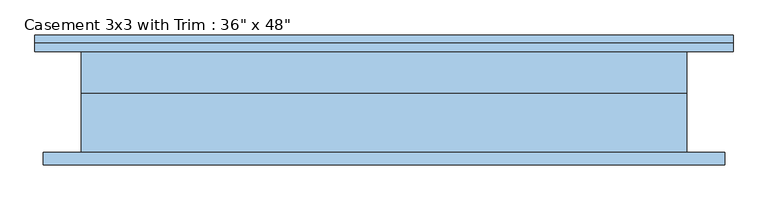
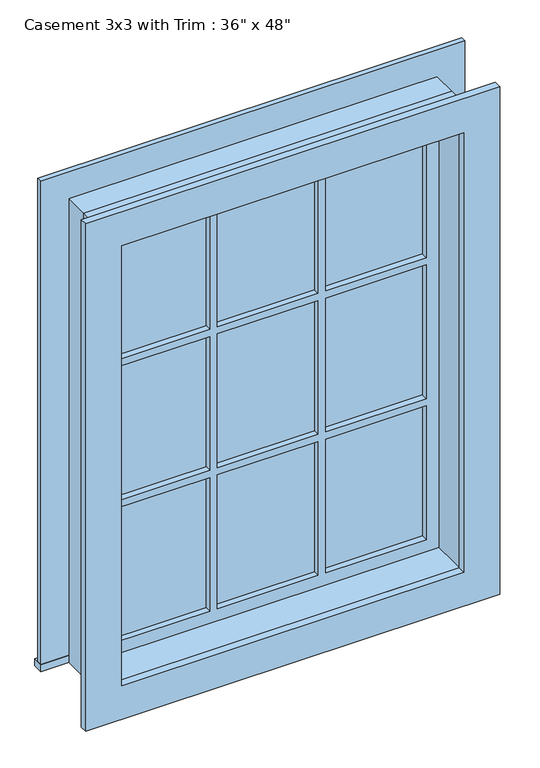
"""IFC4 building model written with IfcOpenShell, lengths in millimetres: window geometry."""

from ifc_helpers import new_model, si_unit, frame, origin, place, context, project, spatial, polyline, outline, extrude, source, transform, mapped, element, save


def window_5c190c7e(model_context):
    return source(origin(), model_context, "Body", "SweptSolid", [
        extrude(outline(polyline([(-527.05, 101.6), (527.05, 101.6), (527.05, 76.2), (-527.05, 76.2), (-527.05, 101.6)])), frame((0.0, 0.0, 914.4), z_axis=(0.0, 0.0, 1.0), x_axis=(1.0, 0.0, 0.0)), (0.0, 0.0, 1.0), 19.05),
        extrude(outline(polyline([(2114.55, -438.15), (2114.55, 438.15), (933.45, 438.15), (933.45, 527.05), (2203.45, 527.05), (2203.45, -527.05), (933.45, -527.05), (933.45, -438.15), (2114.55, -438.15)])), frame((0.0, 76.2, 0.0), z_axis=(0.0, 1.0, 0.0), x_axis=(0.0, 0.0, 1.0)), (0.0, 0.0, 1.0), 12.7),
        extrude(outline(polyline([(143.9333333, 41.275), (393.7, 41.275), (393.7, 28.575), (143.9333333, 28.575), (143.9333333, 41.275)])), frame((0.0, 0.0, 1718.7333333), z_axis=(0.0, 0.0, 1.0), x_axis=(1.0, 0.0, 0.0)), (0.0, 0.0, 1.0), 351.3666667),
        extrude(outline(polyline([(-124.8833333, 41.275), (124.8833333, 41.275), (124.8833333, 28.575), (-124.8833333, 28.575), (-124.8833333, 41.275)])), frame((0.0, 0.0, 1718.7333333), z_axis=(0.0, 0.0, 1.0), x_axis=(1.0, 0.0, 0.0)), (0.0, 0.0, 1.0), 351.3666667),
        extrude(outline(polyline([(-393.7, 41.275), (-143.9333333, 41.275), (-143.9333333, 28.575), (-393.7, 28.575), (-393.7, 41.275)])), frame((0.0, 0.0, 1718.7333333), z_axis=(0.0, 0.0, 1.0), x_axis=(1.0, 0.0, 0.0)), (0.0, 0.0, 1.0), 351.3666667),
        extrude(outline(polyline([(-393.7, 41.275), (-143.9333333, 41.275), (-143.9333333, 28.575), (-393.7, 28.575), (-393.7, 41.275)])), frame((0.0, 0.0, 1348.3166667), z_axis=(0.0, 0.0, 1.0), x_axis=(1.0, 0.0, 0.0)), (0.0, 0.0, 1.0), 351.3666667),
        extrude(outline(polyline([(-124.8833333, 41.275), (124.8833333, 41.275), (124.8833333, 28.575), (-124.8833333, 28.575), (-124.8833333, 41.275)])), frame((0.0, 0.0, 1348.3166667), z_axis=(0.0, 0.0, 1.0), x_axis=(1.0, 0.0, 0.0)), (0.0, 0.0, 1.0), 351.3666667),
        extrude(outline(polyline([(143.9333333, 41.275), (393.7, 41.275), (393.7, 28.575), (143.9333333, 28.575), (143.9333333, 41.275)])), frame((0.0, 0.0, 1348.3166667), z_axis=(0.0, 0.0, 1.0), x_axis=(1.0, 0.0, 0.0)), (0.0, 0.0, 1.0), 351.3666667),
        extrude(outline(polyline([(143.9333333, 41.275), (393.7, 41.275), (393.7, 28.575), (143.9333333, 28.575), (143.9333333, 41.275)])), frame((0.0, 0.0, 977.9), z_axis=(0.0, 0.0, 1.0), x_axis=(1.0, 0.0, 0.0)), (0.0, 0.0, 1.0), 351.3666667),
        extrude(outline(polyline([(-124.8833333, 41.275), (124.8833333, 41.275), (124.8833333, 28.575), (-124.8833333, 28.575), (-124.8833333, 41.275)])), frame((0.0, 0.0, 977.9), z_axis=(0.0, 0.0, 1.0), x_axis=(1.0, 0.0, 0.0)), (0.0, 0.0, 1.0), 351.3666667),
        extrude(outline(polyline([(-393.7, 41.275), (-143.9333333, 41.275), (-143.9333333, 28.575), (-393.7, 28.575), (-393.7, 41.275)])), frame((0.0, 0.0, 977.9), z_axis=(0.0, 0.0, 1.0), x_axis=(1.0, 0.0, 0.0)), (0.0, 0.0, 1.0), 351.3666667),
        extrude(outline(polyline([(2190.75, 514.35), (2190.75, -514.35), (857.25, -514.35), (857.25, 514.35), (2190.75, 514.35)]), holes=[polyline([(2101.85, 425.45), (946.15, 425.45), (946.15, -425.45), (2101.85, -425.45), (2101.85, 425.45)])]), frame((0.0, -95.25, 0.0), z_axis=(0.0, 1.0, 0.0), x_axis=(0.0, 0.0, 1.0)), (0.0, 0.0, 1.0), 19.05),
        extrude(outline(polyline([(2114.55, -438.15), (933.45, -438.15), (933.45, 438.15), (2114.55, 438.15), (2114.55, -438.15)]), holes=[polyline([(2070.1, -143.9333333), (1718.7333333, -143.9333333), (1718.7333333, -393.7), (2070.1, -393.7), (2070.1, -143.9333333)]), polyline([(1699.6833333, -143.9333333), (1348.3166667, -143.9333333), (1348.3166667, -393.7), (1699.6833333, -393.7), (1699.6833333, -143.9333333)]), polyline([(1329.2666667, -143.9333333), (977.9, -143.9333333), (977.9, -393.7), (1329.2666667, -393.7), (1329.2666667, -143.9333333)]), polyline([(2070.1, 124.8833333), (1718.7333333, 124.8833333), (1718.7333333, -124.8833333), (2070.1, -124.8833333), (2070.1, 124.8833333)]), polyline([(1699.6833333, 124.8833333), (1348.3166667, 124.8833333), (1348.3166667, -124.8833333), (1699.6833333, -124.8833333), (1699.6833333, 124.8833333)]), polyline([(1329.2666667, 124.8833333), (977.9, 124.8833333), (977.9, -124.8833333), (1329.2666667, -124.8833333), (1329.2666667, 124.8833333)]), polyline([(2070.1, 393.7), (1718.7333333, 393.7), (1718.7333333, 143.9333333), (2070.1, 143.9333333), (2070.1, 393.7)]), polyline([(1699.6833333, 393.7), (1348.3166667, 393.7), (1348.3166667, 143.9333333), (1699.6833333, 143.9333333), (1699.6833333, 393.7)]), polyline([(1329.2666667, 393.7), (977.9, 393.7), (977.9, 143.9333333), (1329.2666667, 143.9333333), (1329.2666667, 393.7)])]), frame((0.0, 12.7, 0.0), z_axis=(0.0, 1.0, 0.0), x_axis=(0.0, 0.0, 1.0)), (0.0, 0.0, 1.0), 44.45),
        extrude(outline(polyline([(2133.6, -457.2), (914.4, -457.2), (914.4, 457.2), (2133.6, 457.2), (2133.6, -457.2)]), holes=[polyline([(2101.85, -425.45), (2101.85, 425.45), (946.15, 425.45), (946.15, -425.45), (2101.85, -425.45)])]), frame((0.0, -76.2, 0.0), z_axis=(0.0, 1.0, 0.0), x_axis=(0.0, 0.0, 1.0)), (0.0, 0.0, 1.0), 88.9),
        extrude(outline(polyline([(2133.6, 457.2), (2133.6, -457.2), (914.4, -457.2), (914.4, 457.2), (2133.6, 457.2)]), holes=[polyline([(2114.55, 438.15), (933.45, 438.15), (933.45, -438.15), (2114.55, -438.15), (2114.55, 438.15)])]), frame((0.0, 12.7, 0.0), z_axis=(0.0, 1.0, 0.0), x_axis=(0.0, 0.0, 1.0)), (0.0, 0.0, 1.0), 63.5),
    ])


if __name__ == "__main__":
    model = new_model("IFC4")
    model_context = context("Model", 3, world=origin())
    ifc_project = project(units=[si_unit("LENGTHUNIT", "METRE", prefix="MILLI")], contexts=[model_context])
    site = spatial("IfcSite", under=ifc_project)
    building = spatial("IfcBuilding", under=site)
    placement = place(None, origin())
    window_shape = window_5c190c7e(model_context)
    element("IfcWindow", 1, ObjectType="Casement 3x3 with Trim : 36\" x 48\"", at=placement, inside=building, context=model_context, shape_type="MappedRepresentation", body=[
        mapped(window_shape, transform((0.0, 0.0, 0.0), x_axis=(1.0, 0.0, 0.0), y_axis=(0.0, 1.0, 0.0), z_axis=(0.0, 0.0, 1.0))),
    ])
    save(model, "model.ifc")

# Revit data of these elements
# Type "Casement 3x3 with Trim : 36\" x 48\""
#   Type Mark = "20"
#   Construction Type Id = "GSP4R"
#   Assembly Code = "B2020100"
#   Analytic Construction = "1/8 in Pilkington single glazing"
#   Visual Light Transmittance = 0.9
#   Solar Heat Gain Coefficient = 0.78
#   Heat Transfer Coefficient (U) = 0.6496 BTU/(h·ft²·°F)
#   Height = 4' - 0"
#   Default Sill Height = 3' - 0"
#   Trim Projection - Ext. = 0' - 0 1/2"
#   Trim Projection - Int. = 0' - 0 3/4"
#   Trim Width - Exterior = 0' - 3 1/2"
#   Trim Width - Interior = 0' - 3 1/2"
#   Width = 3' - 0"
#   Window Inset = 0' - 0 3/4"
#   Define Thermal Properties by = 1
#   Glass Pane Material = Glass
#   Sash Material = Sash
#   Trim Exterior Material = Trim
#   Trim Interior Material = Trim
#   Wall Closure = (empty or 0)
# Element 1 (IfcWindow, "Casement 3x3 with Trim : 36\" x 48\"")
#   Materials on its faces: "Sash", "Glass", "Trim"
# Materials
#   "Glass": class "Glass", colour RGB 0 128 192, transparency 0.75, Description = "Soda Lime Glass", Cost = 0
#   "Sash": class "Wood", colour RGB 224 178 126, transparency 0
#   "Trim": class "Wood", colour RGB 224 178 126, transparency 0
